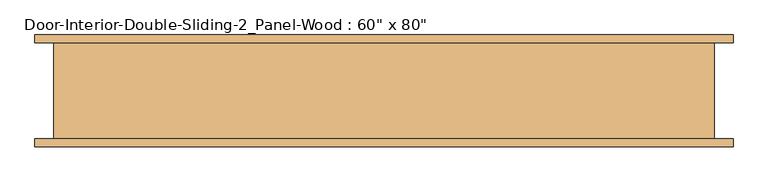
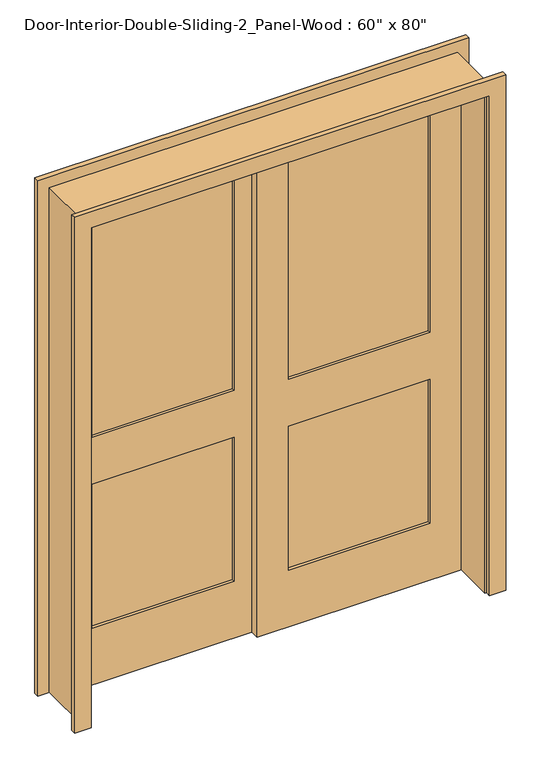
"""IFC4 building model written with IfcOpenShell, lengths in millimetres: door geometry."""

from ifc_helpers import new_model, si_unit, frame, origin, place, context, project, spatial, polyline, outline, extrude, source, transform, mapped, element, save


def door_61c74ce0(model_context):
    return source(origin(), model_context, "Body", "SweptSolid", [
        extrude(outline(polyline([(641.35, 52.9166667), (95.25, 52.9166667), (95.25, 64.5583333), (641.35, 64.5583333), (641.35, 52.9166667)])), frame((0.0, 0.0, 1009.65), z_axis=(0.0, 0.0, 1.0), x_axis=(1.0, 0.0, 0.0)), (0.0, 0.0, 1.0), 903.2875),
        extrude(outline(polyline([(641.35, 52.9166667), (95.25, 52.9166667), (95.25, 64.5583333), (641.35, 64.5583333), (641.35, 52.9166667)])), frame((0.0, 0.0, 231.775), z_axis=(0.0, 0.0, 1.0), x_axis=(1.0, 0.0, 0.0)), (0.0, 0.0, 1.0), 587.375),
        extrude(outline(polyline([(2032.0, -25.4), (0.0, -25.4), (0.0, 762.0), (2032.0, 762.0), (2032.0, -25.4)]), holes=[polyline([(1912.9375, 95.25), (1912.9375, 641.35), (1009.65, 641.35), (1009.65, 95.25), (1912.9375, 95.25)]), polyline([(819.15, 95.25), (819.15, 641.35), (231.775, 641.35), (231.775, 95.25), (819.15, 95.25)])]), frame((0.0, 41.275, 0.0), z_axis=(0.0, 1.0, 0.0), x_axis=(0.0, 0.0, 1.0)), (0.0, 0.0, 1.0), 34.925),
        extrude(outline(polyline([(-95.25, 87.8416667), (-641.35, 87.8416667), (-641.35, 99.4833333), (-95.25, 99.4833333), (-95.25, 87.8416667)])), frame((0.0, 0.0, 1009.65), z_axis=(0.0, 0.0, 1.0), x_axis=(1.0, 0.0, 0.0)), (0.0, 0.0, 1.0), 903.2875),
        extrude(outline(polyline([(-95.25, 87.8416667), (-641.35, 87.8416667), (-641.35, 99.4833333), (-95.25, 99.4833333), (-95.25, 87.8416667)])), frame((0.0, 0.0, 231.775), z_axis=(0.0, 0.0, 1.0), x_axis=(1.0, 0.0, 0.0)), (0.0, 0.0, 1.0), 587.375),
        extrude(outline(polyline([(2032.0, -762.0), (0.0, -762.0), (0.0, 25.4), (2032.0, 25.4), (2032.0, -762.0)]), holes=[polyline([(1912.9375, -641.35), (1912.9375, -95.25), (1009.65, -95.25), (1009.65, -641.35), (1912.9375, -641.35)]), polyline([(819.15, -641.35), (819.15, -95.25), (231.775, -95.25), (231.775, -641.35), (819.15, -641.35)])]), frame((0.0, 76.2, 0.0), z_axis=(0.0, 1.0, 0.0), x_axis=(0.0, 0.0, 1.0)), (0.0, 0.0, 1.0), 34.925),
        extrude(outline(polyline([(0.0, 762.0), (0.0, 787.4), (2057.4, 787.4), (2057.4, -787.4), (0.0, -787.4), (0.0, -762.0), (2032.0, -762.0), (2032.0, 762.0), (0.0, 762.0)])), frame((0.0, -117.475, 0.0), z_axis=(0.0, 1.0, 0.0), x_axis=(0.0, 0.0, 1.0)), (0.0, 0.0, 1.0), 228.6),
        extrude(outline(polyline([(0.0, 768.35), (0.0, 831.85), (2101.85, 831.85), (2101.85, -831.85), (0.0, -831.85), (0.0, -768.35), (2038.35, -768.35), (2038.35, 768.35), (0.0, 768.35)])), frame((0.0, -136.525, 0.0), z_axis=(0.0, 1.0, 0.0), x_axis=(0.0, 0.0, 1.0)), (0.0, 0.0, 1.0), 19.05),
        extrude(outline(polyline([(0.0, 768.35), (0.0, 831.85), (2101.85, 831.85), (2101.85, -831.85), (0.0, -831.85), (0.0, -768.35), (2038.35, -768.35), (2038.35, 768.35), (0.0, 768.35)])), frame((0.0, 111.125, 0.0), z_axis=(0.0, 1.0, 0.0), x_axis=(0.0, 0.0, 1.0)), (0.0, 0.0, 1.0), 19.05),
    ])


if __name__ == "__main__":
    model = new_model("IFC4")
    model_context = context("Model", 3, world=origin())
    ifc_project = project(units=[si_unit("LENGTHUNIT", "METRE", prefix="MILLI")], contexts=[model_context])
    site = spatial("IfcSite", under=ifc_project)
    building = spatial("IfcBuilding", under=site)
    placement = place(None, origin())
    door_shape = door_61c74ce0(model_context)
    element("IfcDoor", 1, ObjectType="Door-Interior-Double-Sliding-2_Panel-Wood : 60\" x 80\"", at=placement, inside=building, context=model_context, shape_type="MappedRepresentation", body=[
        mapped(door_shape, transform((0.0, 0.0, 0.0), x_axis=(1.0, 0.0, 0.0), y_axis=(0.0, 1.0, 0.0), z_axis=(0.0, 0.0, 1.0))),
    ])
    save(model, "model.ifc")

# Revit data of these elements
# Type "Door-Interior-Double-Sliding-2_Panel-Wood : 60\" x 80\""
#   Type Mark = "8"
#   Assembly Code = "C1020300"
#   Analytic Construction = "Wooden"
#   Top Rail = 0' - 4 11/16"
#   Thickness = 0' - 1 3/8"
#   Thermal Resistance (R) = 2.5876 (h·ft²·°F)/BTU
#   Stiles = 0' - 4 3/4"
#   Rough Width = 5' - 2"
#   Rough Height = 6' - 9"
#   Lock Rail = 0' - 7 1/2"
#   Height = 6' - 8"
#   Width = 5' - 0"
#   Heat Transfer Coefficient (U) = 0.3865 BTU/(h·ft²·°F)
#   Bottom Rail = 0' - 9 1/8"
#   Trim Material = Cherry
#   Panel Material = Cherry
#   Frame Material = Cherry
#   Visual Light Transmittance = 0
#   Solar Heat Gain Coefficient = 0
#   Wall Closure = (empty or 0)
#   Function = (empty or 0)
# Element 1 (IfcDoor, "Door-Interior-Double-Sliding-2_Panel-Wood : 60\" x 80\"")
#   Materials on its faces: "Cherry"
# Materials
#   "Cherry": class "Wood", colour RGB 226 177 128, transparency 0, Description = "Prunus Serotina", Cost = 0
